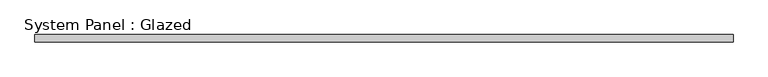
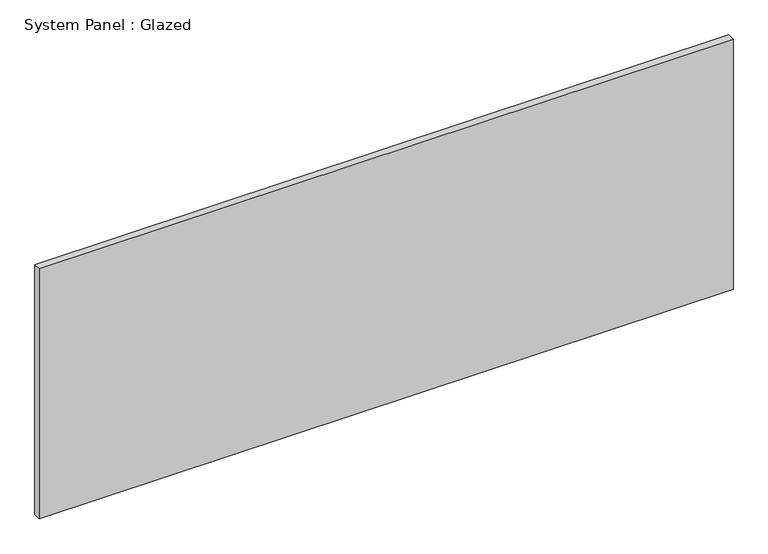
"""IFC4 building model written with IfcOpenShell, lengths in millimetres: plate geometry, System Panel : Glazed."""

from ifc_helpers import new_model, si_unit, origin, origin_with_axes, place, context, project, spatial, polyline, outline, extrude, source, transform, mapped, element, save


def system_panel_glazed_361f77d3(model_context):
    return source(origin(), model_context, "Body", "SweptSolid", [
        extrude(outline(polyline([(1208.9721298, 19.05), (-1208.9721298, 19.05), (-1208.9721298, 44.45), (1208.9721298, 44.45), (1208.9721298, 19.05)])), origin_with_axes(), (0.0, 0.0, 1.0), 920.9396511),
    ])


if __name__ == "__main__":
    model = new_model("IFC4")
    model_context = context("Model", 3, world=origin())
    ifc_project = project(units=[si_unit("LENGTHUNIT", "METRE", prefix="MILLI")], contexts=[model_context])
    site = spatial("IfcSite", under=ifc_project)
    building = spatial("IfcBuilding", under=site)
    placement = place(None, origin())
    system_panel_glazed_shape = system_panel_glazed_361f77d3(model_context)
    element("IfcPlate", 1, ObjectType="System Panel : Glazed", at=placement, inside=building, context=model_context, shape_type="MappedRepresentation", body=[
        mapped(system_panel_glazed_shape, transform((0.0, 0.0, 0.0), x_axis=(1.0, 0.0, 0.0), y_axis=(0.0, 1.0, 0.0), z_axis=(0.0, 0.0, 1.0))),
    ])
    save(model, "model.ifc")

# Revit data of these elements
# Type "System Panel : Glazed"
#   Construction Type Id = "GSP4R"
#   Analytic Construction = "1/8 in Pilkington single glazing"
#   Visual Light Transmittance = 0.9
#   Solar Heat Gain Coefficient = 0.86
#   Heat Transfer Coefficient (U) = 1.18115 BTU/(h·ft²·°F)
#   Define Thermal Properties by = 1
# Element 1 (IfcPlate, "System Panel : Glazed")
#   Materials on its faces: "Glass"
# Materials
#   "Glass": class "Glass", colour RGB 0 128 192, transparency 0.75, Description = "Soda Lime Glass", Cost = 0
